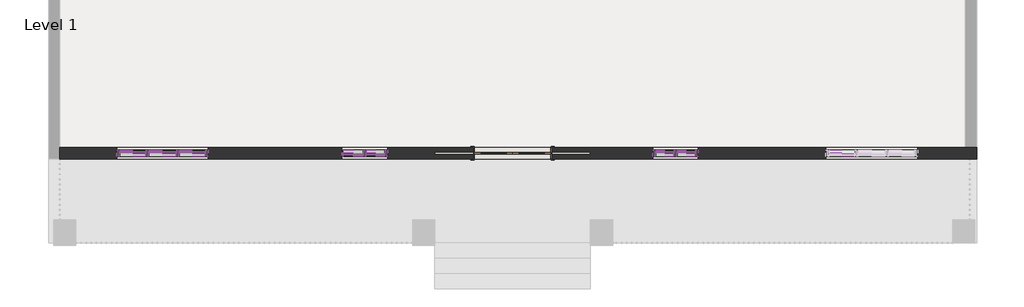
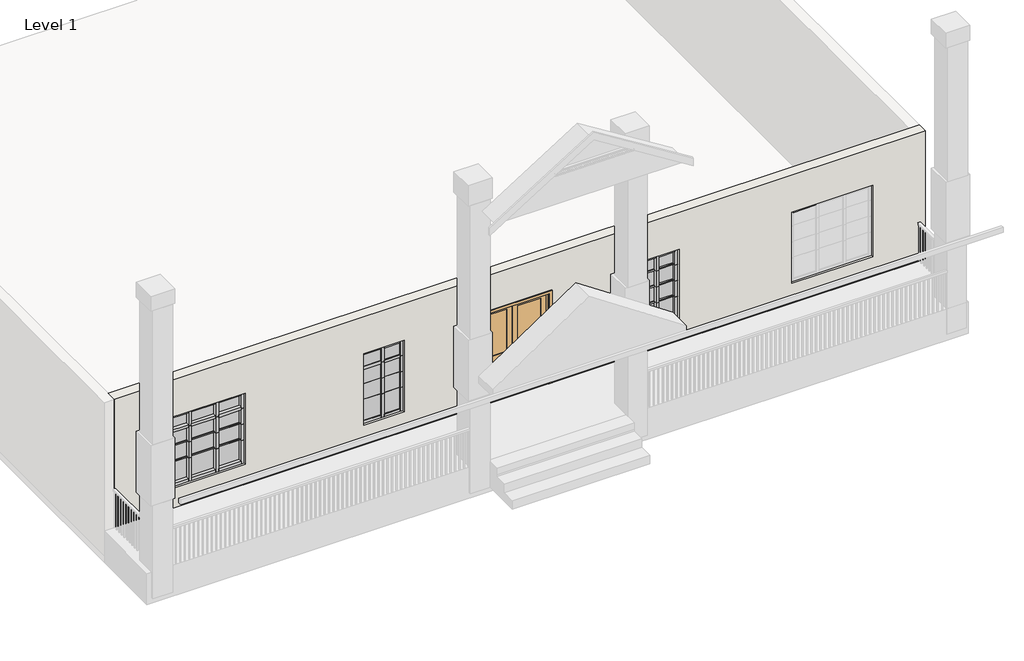
# One storey, part 1 of 3: 79 members, 28 plates, 1 door, 1 wall.
"""IFC4 building model written with IfcOpenShell, lengths in millimetres."""

from ifc_helpers import new_model, si_unit, origin, place, context, project, spatial, faceted_brep, transform, mapped, element, save
from components import door_7a66d0d1, member_34aa1075, member_9625144b, member_80fbcd94, member_5d13e7fd, member_2344d604, member_b1407fb7, member_31f2b2ad, member_0b7646a3, member_bc554fa6, member_aaa03826, member_0a1a1ade, member_a980948f, member_03a502dc, member_dfe75557, member_50cacee6, member_1ad5418d, member_843225dc, member_6103f85b, member_af2f84b9, member_d2340509, member_8fd572c7, member_8d9b4452, member_6f432376, system_panel_glazed_6026b5c4, system_panel_glazed_0f474f61, system_panel_glazed_5422c98d, system_panel_glazed_c61bacb6, system_panel_glazed_055f9577, system_panel_glazed_5ecf2d74, system_panel_glazed_969e6b50, system_panel_glazed_86de8a05, system_panel_glazed_a58f4d23, system_panel_glazed_6b1abce8, system_panel_glazed_499f07c7, system_panel_glazed_73771f90, system_panel_glazed_6a2c27ee, system_panel_glazed_d5759347, system_panel_glazed_b1e52c84, system_panel_glazed_6ee44b12, system_panel_glazed_6c61ac18, system_panel_glazed_c76c6b52, system_panel_glazed_5d34ab6a

model = new_model("IFC4")

# Units and contexts
model_context = context("Model", 3, world=origin())
ifc_project = project(units=[si_unit("LENGTHUNIT", "METRE", prefix="MILLI")], contexts=[model_context])

# Site, building, storey
site = spatial("IfcSite", under=ifc_project)
building = spatial("IfcBuilding", under=site)
storey = spatial("IfcBuildingStorey", under=building, Name="Level 1", Elevation=0.0)

# Door
placement = place(None, origin())
door_shape = door_7a66d0d1(model_context)
element("IfcDoor", 1, ObjectType="Door-Interior-Double-Pocket-2_Panel-Wood : 60\" x 84\"", at=placement, inside=storey, context=model_context, shape_type="MappedRepresentation", body=[
    mapped(door_shape, transform((-512.1420659, -6986.1878342, 609.6), x_axis=(1.0, 0.0, 0.0), y_axis=(0.0, 1.0, 0.0), z_axis=(0.0, 0.0, 1.0))),
])

# Members
member_shape = member_34aa1075(model_context)
element("IfcMember", 2, ObjectType="Rectangular Mullion : 1\" Square", at=placement, inside=storey, context=model_context, shape_type="MappedRepresentation", body=[
    mapped(member_shape, transform((-3917.6050805, -6986.1878342, 1631.95), x_axis=(-1.0, 0.0, 0.0), y_axis=(0.0, 1.0, 0.0), z_axis=(0.0, 0.0, -1.0))),
])
member_2_shape = member_9625144b(model_context)
element("IfcMember", 3, ObjectType="Rectangular Mullion : 1\" Square", at=placement, inside=storey, context=model_context, shape_type="MappedRepresentation", body=[
    mapped(member_2_shape, transform((-6646.2420659, -6986.1878342, 2006.6), x_axis=(0.0, 0.0, 1.0), y_axis=(0.0, -1.0, 0.0), z_axis=(1.0, 0.0, 0.0))),
])
element("IfcMember", 4, ObjectType="Rectangular Mullion : 1\" Square", at=placement, inside=storey, context=model_context, shape_type="MappedRepresentation", body=[
    mapped(member_2_shape, transform((-7833.6920659, -6986.1878342, 2006.6), x_axis=(0.0, 0.0, 1.0), y_axis=(0.0, -1.0, 0.0), z_axis=(1.0, 0.0, 0.0))),
])
element("IfcMember", 5, ObjectType="Rectangular Mullion : 1\" Square", at=placement, inside=storey, context=model_context, shape_type="MappedRepresentation", body=[
    mapped(member_2_shape, transform((-6646.2420659, -6986.1878342, 1625.6), x_axis=(0.0, 0.0, 1.0), y_axis=(0.0, -1.0, 0.0), z_axis=(1.0, 0.0, 0.0))),
])
element("IfcMember", 6, ObjectType="Rectangular Mullion : 1\" Square", at=placement, inside=storey, context=model_context, shape_type="MappedRepresentation", body=[
    mapped(member_2_shape, transform((-7833.6920659, -6986.1878342, 1625.6), x_axis=(0.0, 0.0, 1.0), y_axis=(0.0, -1.0, 0.0), z_axis=(1.0, 0.0, 0.0))),
])
element("IfcMember", 7, ObjectType="Rectangular Mullion : 1\" Square", at=placement, inside=storey, context=model_context, shape_type="MappedRepresentation", body=[
    mapped(member_2_shape, transform((5799.7579341, -6986.1878342, 2006.6), x_axis=(0.0, 0.0, 1.0), y_axis=(0.0, 1.0, 0.0), z_axis=(-1.0, 0.0, 0.0))),
])
element("IfcMember", 8, ObjectType="Rectangular Mullion : 1\" Square", at=placement, inside=storey, context=model_context, shape_type="MappedRepresentation", body=[
    mapped(member_2_shape, transform((5799.7579341, -6986.1878342, 1625.6), x_axis=(0.0, 0.0, 1.0), y_axis=(0.0, 1.0, 0.0), z_axis=(-1.0, 0.0, 0.0))),
])
element("IfcMember", 9, ObjectType="Rectangular Mullion : 1\" Square", at=placement, inside=storey, context=model_context, shape_type="MappedRepresentation", body=[
    mapped(member_2_shape, transform((5799.7579341, -6986.1878342, 2387.6), x_axis=(0.0, 0.0, 1.0), y_axis=(0.0, 1.0, 0.0), z_axis=(-1.0, 0.0, 0.0))),
])
member_3_shape = member_80fbcd94(model_context)
element("IfcMember", 10, ObjectType="Rectangular Mullion : 1\" Square", at=placement, inside=storey, context=model_context, shape_type="MappedRepresentation", body=[
    mapped(member_3_shape, transform((-7224.0920659, -6986.1878342, 2006.6), x_axis=(0.0, 0.0, 1.0), y_axis=(0.0, -1.0, 0.0), z_axis=(1.0, 0.0, 0.0))),
])
element("IfcMember", 11, ObjectType="Rectangular Mullion : 1\" Square", at=placement, inside=storey, context=model_context, shape_type="MappedRepresentation", body=[
    mapped(member_3_shape, transform((-7224.0920659, -6986.1878342, 1625.6), x_axis=(0.0, 0.0, 1.0), y_axis=(0.0, -1.0, 0.0), z_axis=(1.0, 0.0, 0.0))),
])
member_4_shape = member_5d13e7fd(model_context)
element("IfcMember", 12, ObjectType="Rectangular Mullion : 1\" Square", at=placement, inside=storey, context=model_context, shape_type="MappedRepresentation", body=[
    mapped(member_4_shape, transform((-3892.2050805, -6986.1878342, 2006.6), x_axis=(0.0, 0.0, 1.0), y_axis=(0.0, 1.0, 0.0), z_axis=(-1.0, 0.0, 0.0))),
])
element("IfcMember", 13, ObjectType="Rectangular Mullion : 1\" Square", at=placement, inside=storey, context=model_context, shape_type="MappedRepresentation", body=[
    mapped(member_4_shape, transform((-3892.2050805, -6986.1878342, 1631.95), x_axis=(0.0, 0.0, 1.0), y_axis=(0.0, 1.0, 0.0), z_axis=(-1.0, 0.0, 0.0))),
])
member_5_shape = member_2344d604(model_context)
element("IfcMember", 14, ObjectType="Rectangular Mullion : 1\" Square", at=placement, inside=storey, context=model_context, shape_type="MappedRepresentation", body=[
    mapped(member_5_shape, transform((-3428.6550805, -6986.1878342, 2006.6), x_axis=(0.0, 0.0, 1.0), y_axis=(0.0, 1.0, 0.0), z_axis=(-1.0, 0.0, 0.0))),
])
element("IfcMember", 15, ObjectType="Rectangular Mullion : 1\" Square", at=placement, inside=storey, context=model_context, shape_type="MappedRepresentation", body=[
    mapped(member_5_shape, transform((-3428.6550805, -6986.1878342, 1631.95), x_axis=(0.0, 0.0, 1.0), y_axis=(0.0, 1.0, 0.0), z_axis=(-1.0, 0.0, 0.0))),
])
element("IfcMember", 16, ObjectType="Rectangular Mullion : 1\" Square", at=placement, inside=storey, context=model_context, shape_type="MappedRepresentation", body=[
    mapped(member_5_shape, transform((3130.8949195, -6986.1878342, 2387.6), x_axis=(0.0, 0.0, 1.0), y_axis=(0.0, -1.0, 0.0), z_axis=(1.0, 0.0, 0.0))),
])
element("IfcMember", 17, ObjectType="Rectangular Mullion : 1\" Square", at=placement, inside=storey, context=model_context, shape_type="MappedRepresentation", body=[
    mapped(member_5_shape, transform((2705.4449195, -6986.1878342, 2387.6), x_axis=(0.0, 0.0, 1.0), y_axis=(0.0, -1.0, 0.0), z_axis=(1.0, 0.0, 0.0))),
])
element("IfcMember", 18, ObjectType="Rectangular Mullion : 1\" Square", at=placement, inside=storey, context=model_context, shape_type="MappedRepresentation", body=[
    mapped(member_5_shape, transform((3130.8949195, -6986.1878342, 2006.6), x_axis=(0.0, 0.0, 1.0), y_axis=(0.0, -1.0, 0.0), z_axis=(1.0, 0.0, 0.0))),
])
element("IfcMember", 19, ObjectType="Rectangular Mullion : 1\" Square", at=placement, inside=storey, context=model_context, shape_type="MappedRepresentation", body=[
    mapped(member_5_shape, transform((2705.4449195, -6986.1878342, 2006.6), x_axis=(0.0, 0.0, 1.0), y_axis=(0.0, -1.0, 0.0), z_axis=(1.0, 0.0, 0.0))),
])
element("IfcMember", 20, ObjectType="Rectangular Mullion : 1\" Square", at=placement, inside=storey, context=model_context, shape_type="MappedRepresentation", body=[
    mapped(member_5_shape, transform((3130.8949195, -6986.1878342, 1625.6), x_axis=(0.0, 0.0, 1.0), y_axis=(0.0, -1.0, 0.0), z_axis=(1.0, 0.0, 0.0))),
])
element("IfcMember", 21, ObjectType="Rectangular Mullion : 1\" Square", at=placement, inside=storey, context=model_context, shape_type="MappedRepresentation", body=[
    mapped(member_5_shape, transform((2705.4449195, -6986.1878342, 1625.6), x_axis=(0.0, 0.0, 1.0), y_axis=(0.0, -1.0, 0.0), z_axis=(1.0, 0.0, 0.0))),
])
member_6_shape = member_b1407fb7(model_context)
element("IfcMember", 22, ObjectType="Rectangular Mullion : 1\" Square", at=placement, inside=storey, context=model_context, shape_type="MappedRepresentation", body=[
    mapped(member_6_shape, transform((-3917.6050805, -6986.1878342, 2006.6), x_axis=(-1.0, 0.0, 0.0), y_axis=(0.0, 1.0, 0.0), z_axis=(0.0, 0.0, -1.0))),
])
element("IfcMember", 23, ObjectType="Rectangular Mullion : 1\" Square", at=placement, inside=storey, context=model_context, shape_type="MappedRepresentation", body=[
    mapped(member_6_shape, transform((-3917.6050805, -6986.1878342, 2387.6), x_axis=(-1.0, 0.0, 0.0), y_axis=(0.0, 1.0, 0.0), z_axis=(0.0, 0.0, -1.0))),
])
member_7_shape = member_31f2b2ad(model_context)
element("IfcMember", 24, ObjectType="Rectangular Mullion : 1\" Square", at=placement, inside=storey, context=model_context, shape_type="MappedRepresentation", body=[
    mapped(member_7_shape, transform((-3917.6050805, -6986.1878342, 1066.8), x_axis=(-1.0, 0.0, 0.0), y_axis=(0.0, 1.0, 0.0), z_axis=(0.0, 0.0, -1.0))),
])
member_8_shape = member_0b7646a3(model_context)
element("IfcMember", 25, ObjectType="Rectangular Mullion : 2.5\" x 5\" rectangular", at=placement, inside=storey, context=model_context, shape_type="MappedRepresentation", body=[
    mapped(member_8_shape, transform((-6646.2420659, -6986.1878342, 2768.6), x_axis=(0.0, 0.0, 1.0), y_axis=(0.0, -1.0, 0.0), z_axis=(1.0, 0.0, 0.0))),
])
element("IfcMember", 26, ObjectType="Rectangular Mullion : 2.5\" x 5\" rectangular", at=placement, inside=storey, context=model_context, shape_type="MappedRepresentation", body=[
    mapped(member_8_shape, transform((-7833.6920659, -6986.1878342, 2768.6), x_axis=(0.0, 0.0, 1.0), y_axis=(0.0, -1.0, 0.0), z_axis=(1.0, 0.0, 0.0))),
])
element("IfcMember", 27, ObjectType="Rectangular Mullion : 2.5\" x 5\" rectangular", at=placement, inside=storey, context=model_context, shape_type="MappedRepresentation", body=[
    mapped(member_8_shape, transform((5799.7579341, -6986.1878342, 2768.6), x_axis=(0.0, 0.0, 1.0), y_axis=(0.0, 1.0, 0.0), z_axis=(-1.0, 0.0, 0.0))),
])
element("IfcMember", 28, ObjectType="Rectangular Mullion : 2.5\" x 5\" rectangular", at=placement, inside=storey, context=model_context, shape_type="MappedRepresentation", body=[
    mapped(member_8_shape, transform((-8348.0420659, -6986.1878342, 1066.8), x_axis=(0.0, 0.0, -1.0), y_axis=(0.0, -1.0, 0.0), z_axis=(-1.0, 0.0, 0.0))),
])
element("IfcMember", 29, ObjectType="Rectangular Mullion : 2.5\" x 5\" rectangular", at=placement, inside=storey, context=model_context, shape_type="MappedRepresentation", body=[
    mapped(member_8_shape, transform((-7160.5920659, -6986.1878342, 1066.8), x_axis=(0.0, 0.0, -1.0), y_axis=(0.0, -1.0, 0.0), z_axis=(-1.0, 0.0, 0.0))),
])
member_9_shape = member_bc554fa6(model_context)
element("IfcMember", 30, ObjectType="Rectangular Mullion : 2.5\" x 5\" rectangular", at=placement, inside=storey, context=model_context, shape_type="MappedRepresentation", body=[
    mapped(member_9_shape, transform((-7801.9420659, -6986.1878342, 1066.8), x_axis=(1.0, 0.0, 0.0), y_axis=(0.0, -1.0, 0.0), z_axis=(0.0, 0.0, -1.0))),
])
element("IfcMember", 31, ObjectType="Rectangular Mullion : 2.5\" x 5\" rectangular", at=placement, inside=storey, context=model_context, shape_type="MappedRepresentation", body=[
    mapped(member_9_shape, transform((-7192.3420659, -6986.1878342, 1066.8), x_axis=(1.0, 0.0, 0.0), y_axis=(0.0, -1.0, 0.0), z_axis=(0.0, 0.0, -1.0))),
])
element("IfcMember", 32, ObjectType="Rectangular Mullion : 2.5\" x 5\" rectangular", at=placement, inside=storey, context=model_context, shape_type="MappedRepresentation", body=[
    mapped(member_9_shape, transform((2737.1949195, -6986.1878342, 1066.8), x_axis=(1.0, 0.0, 0.0), y_axis=(0.0, -1.0, 0.0), z_axis=(0.0, 0.0, -1.0))),
])
member_10_shape = member_aaa03826(model_context)
element("IfcMember", 33, ObjectType="Rectangular Mullion : 2.5\" x 5\" rectangular", at=placement, inside=storey, context=model_context, shape_type="MappedRepresentation", body=[
    mapped(member_10_shape, transform((-7833.6920659, -6986.1878342, 2387.6), x_axis=(0.0, 0.0, 1.0), y_axis=(0.0, -1.0, 0.0), z_axis=(1.0, 0.0, 0.0))),
])
element("IfcMember", 34, ObjectType="Rectangular Mullion : 2.5\" x 5\" rectangular", at=placement, inside=storey, context=model_context, shape_type="MappedRepresentation", body=[
    mapped(member_10_shape, transform((-6646.2420659, -6986.1878342, 2387.6), x_axis=(0.0, 0.0, 1.0), y_axis=(0.0, -1.0, 0.0), z_axis=(1.0, 0.0, 0.0))),
])
member_11_shape = member_0a1a1ade(model_context)
element("IfcMember", 35, ObjectType="Rectangular Mullion : 2.5\" x 5\" rectangular", at=placement, inside=storey, context=model_context, shape_type="MappedRepresentation", body=[
    mapped(member_11_shape, transform((-7224.0920659, -6986.1878342, 2387.6), x_axis=(0.0, 0.0, 1.0), y_axis=(0.0, -1.0, 0.0), z_axis=(1.0, 0.0, 0.0))),
])
member_12_shape = member_a980948f(model_context)
element("IfcMember", 36, ObjectType="Rectangular Mullion : 2.5\" x 5\" rectangular", at=placement, inside=storey, context=model_context, shape_type="MappedRepresentation", body=[
    mapped(member_12_shape, transform((-7770.1920659, -6986.1878342, 1066.8), x_axis=(0.0, 0.0, -1.0), y_axis=(0.0, -1.0, 0.0), z_axis=(-1.0, 0.0, 0.0))),
])
element("IfcMember", 37, ObjectType="Rectangular Mullion : 2.5\" x 5\" rectangular", at=placement, inside=storey, context=model_context, shape_type="MappedRepresentation", body=[
    mapped(member_12_shape, transform((-7224.0920659, -6986.1878342, 2768.6), x_axis=(0.0, 0.0, 1.0), y_axis=(0.0, -1.0, 0.0), z_axis=(1.0, 0.0, 0.0))),
])
member_13_shape = member_03a502dc(model_context)
element("IfcMember", 38, ObjectType="Rectangular Mullion : 2.5\" x 5\" rectangular", at=placement, inside=storey, context=model_context, shape_type="MappedRepresentation", body=[
    mapped(member_13_shape, transform((-7801.9420659, -6986.1878342, 2387.6), x_axis=(1.0, 0.0, 0.0), y_axis=(0.0, -1.0, 0.0), z_axis=(0.0, 0.0, -1.0))),
])
element("IfcMember", 39, ObjectType="Rectangular Mullion : 2.5\" x 5\" rectangular", at=placement, inside=storey, context=model_context, shape_type="MappedRepresentation", body=[
    mapped(member_13_shape, transform((-7192.3420659, -6986.1878342, 2387.6), x_axis=(1.0, 0.0, 0.0), y_axis=(0.0, -1.0, 0.0), z_axis=(0.0, 0.0, -1.0))),
])
element("IfcMember", 40, ObjectType="Rectangular Mullion : 2.5\" x 5\" rectangular", at=placement, inside=storey, context=model_context, shape_type="MappedRepresentation", body=[
    mapped(member_13_shape, transform((-3460.4050805, -6986.1878342, 2387.6), x_axis=(-1.0, 0.0, 0.0), y_axis=(0.0, 1.0, 0.0), z_axis=(0.0, 0.0, -1.0))),
])
element("IfcMember", 41, ObjectType="Rectangular Mullion : 2.5\" x 5\" rectangular", at=placement, inside=storey, context=model_context, shape_type="MappedRepresentation", body=[
    mapped(member_13_shape, transform((2737.1949195, -6986.1878342, 2387.6), x_axis=(1.0, 0.0, 0.0), y_axis=(0.0, -1.0, 0.0), z_axis=(0.0, 0.0, -1.0))),
])
element("IfcMember", 42, ObjectType="Rectangular Mullion : 2.5\" x 5\" rectangular", at=placement, inside=storey, context=model_context, shape_type="MappedRepresentation", body=[
    mapped(member_13_shape, transform((-7801.9420659, -6986.1878342, 2006.6), x_axis=(1.0, 0.0, 0.0), y_axis=(0.0, -1.0, 0.0), z_axis=(0.0, 0.0, -1.0))),
])
element("IfcMember", 43, ObjectType="Rectangular Mullion : 2.5\" x 5\" rectangular", at=placement, inside=storey, context=model_context, shape_type="MappedRepresentation", body=[
    mapped(member_13_shape, transform((-7801.9420659, -6986.1878342, 1625.6), x_axis=(1.0, 0.0, 0.0), y_axis=(0.0, -1.0, 0.0), z_axis=(0.0, 0.0, -1.0))),
])
element("IfcMember", 44, ObjectType="Rectangular Mullion : 2.5\" x 5\" rectangular", at=placement, inside=storey, context=model_context, shape_type="MappedRepresentation", body=[
    mapped(member_13_shape, transform((-7192.3420659, -6986.1878342, 2006.6), x_axis=(1.0, 0.0, 0.0), y_axis=(0.0, -1.0, 0.0), z_axis=(0.0, 0.0, -1.0))),
])
element("IfcMember", 45, ObjectType="Rectangular Mullion : 2.5\" x 5\" rectangular", at=placement, inside=storey, context=model_context, shape_type="MappedRepresentation", body=[
    mapped(member_13_shape, transform((-7192.3420659, -6986.1878342, 1625.6), x_axis=(1.0, 0.0, 0.0), y_axis=(0.0, -1.0, 0.0), z_axis=(0.0, 0.0, -1.0))),
])
element("IfcMember", 46, ObjectType="Rectangular Mullion : 2.5\" x 5\" rectangular", at=placement, inside=storey, context=model_context, shape_type="MappedRepresentation", body=[
    mapped(member_13_shape, transform((-3460.4050805, -6986.1878342, 2006.6), x_axis=(-1.0, 0.0, 0.0), y_axis=(0.0, 1.0, 0.0), z_axis=(0.0, 0.0, -1.0))),
])
element("IfcMember", 47, ObjectType="Rectangular Mullion : 2.5\" x 5\" rectangular", at=placement, inside=storey, context=model_context, shape_type="MappedRepresentation", body=[
    mapped(member_13_shape, transform((2737.1949195, -6986.1878342, 2006.6), x_axis=(1.0, 0.0, 0.0), y_axis=(0.0, -1.0, 0.0), z_axis=(0.0, 0.0, -1.0))),
])
element("IfcMember", 48, ObjectType="Rectangular Mullion : 2.5\" x 5\" rectangular", at=placement, inside=storey, context=model_context, shape_type="MappedRepresentation", body=[
    mapped(member_13_shape, transform((2737.1949195, -6986.1878342, 1625.6), x_axis=(1.0, 0.0, 0.0), y_axis=(0.0, -1.0, 0.0), z_axis=(0.0, 0.0, -1.0))),
])
member_14_shape = member_dfe75557(model_context)
element("IfcMember", 49, ObjectType="Rectangular Mullion : 2.5\" x 5\" rectangular", at=placement, inside=storey, context=model_context, shape_type="MappedRepresentation", body=[
    mapped(member_14_shape, transform((-8411.5420659, -6986.1878342, 2768.6), x_axis=(-1.0, 0.0, 0.0), y_axis=(0.0, -1.0, 0.0), z_axis=(0.0, 0.0, 1.0))),
])
element("IfcMember", 50, ObjectType="Rectangular Mullion : 2.5\" x 5\" rectangular", at=placement, inside=storey, context=model_context, shape_type="MappedRepresentation", body=[
    mapped(member_14_shape, transform((-3003.2050805, -6986.1878342, 2768.6), x_axis=(1.0, 0.0, 0.0), y_axis=(0.0, 1.0, 0.0), z_axis=(0.0, 0.0, 1.0))),
])
element("IfcMember", 51, ObjectType="Rectangular Mullion : 2.5\" x 5\" rectangular", at=placement, inside=storey, context=model_context, shape_type="MappedRepresentation", body=[
    mapped(member_14_shape, transform((2279.9949195, -6986.1878342, 2768.6), x_axis=(-1.0, 0.0, 0.0), y_axis=(0.0, -1.0, 0.0), z_axis=(0.0, 0.0, 1.0))),
])
member_15_shape = member_50cacee6(model_context)
element("IfcMember", 52, ObjectType="Rectangular Mullion : 2.5\" x 5\" rectangular", at=placement, inside=storey, context=model_context, shape_type="MappedRepresentation", body=[
    mapped(member_15_shape, transform((-6582.7420659, -6986.1878342, 1066.8), x_axis=(1.0, 0.0, 0.0), y_axis=(0.0, -1.0, 0.0), z_axis=(0.0, 0.0, -1.0))),
])
element("IfcMember", 53, ObjectType="Rectangular Mullion : 2.5\" x 5\" rectangular", at=placement, inside=storey, context=model_context, shape_type="MappedRepresentation", body=[
    mapped(member_15_shape, transform((3194.3949195, -6986.1878342, 1066.8), x_axis=(1.0, 0.0, 0.0), y_axis=(0.0, -1.0, 0.0), z_axis=(0.0, 0.0, -1.0))),
])
element("IfcMember", 54, ObjectType="Rectangular Mullion : 2.5\" x 5\" rectangular", at=placement, inside=storey, context=model_context, shape_type="MappedRepresentation", body=[
    mapped(member_14_shape, transform((-6582.7420659, -6986.1878342, 2387.6), x_axis=(1.0, 0.0, 0.0), y_axis=(0.0, -1.0, 0.0), z_axis=(0.0, 0.0, -1.0))),
])
element("IfcMember", 55, ObjectType="Rectangular Mullion : 2.5\" x 5\" rectangular", at=placement, inside=storey, context=model_context, shape_type="MappedRepresentation", body=[
    mapped(member_14_shape, transform((3194.3949195, -6986.1878342, 2387.6), x_axis=(1.0, 0.0, 0.0), y_axis=(0.0, -1.0, 0.0), z_axis=(0.0, 0.0, -1.0))),
])
element("IfcMember", 56, ObjectType="Rectangular Mullion : 2.5\" x 5\" rectangular", at=placement, inside=storey, context=model_context, shape_type="MappedRepresentation", body=[
    mapped(member_14_shape, transform((-6582.7420659, -6986.1878342, 2006.6), x_axis=(1.0, 0.0, 0.0), y_axis=(0.0, -1.0, 0.0), z_axis=(0.0, 0.0, -1.0))),
])
element("IfcMember", 57, ObjectType="Rectangular Mullion : 2.5\" x 5\" rectangular", at=placement, inside=storey, context=model_context, shape_type="MappedRepresentation", body=[
    mapped(member_14_shape, transform((-6582.7420659, -6986.1878342, 1625.6), x_axis=(1.0, 0.0, 0.0), y_axis=(0.0, -1.0, 0.0), z_axis=(0.0, 0.0, -1.0))),
])
element("IfcMember", 58, ObjectType="Rectangular Mullion : 2.5\" x 5\" rectangular", at=placement, inside=storey, context=model_context, shape_type="MappedRepresentation", body=[
    mapped(member_14_shape, transform((3194.3949195, -6986.1878342, 2006.6), x_axis=(1.0, 0.0, 0.0), y_axis=(0.0, -1.0, 0.0), z_axis=(0.0, 0.0, -1.0))),
])
element("IfcMember", 59, ObjectType="Rectangular Mullion : 2.5\" x 5\" rectangular", at=placement, inside=storey, context=model_context, shape_type="MappedRepresentation", body=[
    mapped(member_14_shape, transform((3194.3949195, -6986.1878342, 1625.6), x_axis=(1.0, 0.0, 0.0), y_axis=(0.0, -1.0, 0.0), z_axis=(0.0, 0.0, -1.0))),
])
element("IfcMember", 60, ObjectType="Rectangular Mullion : 2.5\" x 5\" rectangular", at=placement, inside=storey, context=model_context, shape_type="MappedRepresentation", body=[
    mapped(member_14_shape, transform((-8411.5420659, -6986.1878342, 2387.6), x_axis=(-1.0, 0.0, 0.0), y_axis=(0.0, -1.0, 0.0), z_axis=(0.0, 0.0, 1.0))),
])
element("IfcMember", 61, ObjectType="Rectangular Mullion : 2.5\" x 5\" rectangular", at=placement, inside=storey, context=model_context, shape_type="MappedRepresentation", body=[
    mapped(member_14_shape, transform((-8411.5420659, -6986.1878342, 2006.6), x_axis=(-1.0, 0.0, 0.0), y_axis=(0.0, -1.0, 0.0), z_axis=(0.0, 0.0, 1.0))),
])
element("IfcMember", 62, ObjectType="Rectangular Mullion : 2.5\" x 5\" rectangular", at=placement, inside=storey, context=model_context, shape_type="MappedRepresentation", body=[
    mapped(member_14_shape, transform((-3003.2050805, -6986.1878342, 2387.6), x_axis=(1.0, 0.0, 0.0), y_axis=(0.0, 1.0, 0.0), z_axis=(0.0, 0.0, 1.0))),
])
element("IfcMember", 63, ObjectType="Rectangular Mullion : 2.5\" x 5\" rectangular", at=placement, inside=storey, context=model_context, shape_type="MappedRepresentation", body=[
    mapped(member_14_shape, transform((2279.9949195, -6986.1878342, 2387.6), x_axis=(-1.0, 0.0, 0.0), y_axis=(0.0, -1.0, 0.0), z_axis=(0.0, 0.0, 1.0))),
])
element("IfcMember", 64, ObjectType="Rectangular Mullion : 2.5\" x 5\" rectangular", at=placement, inside=storey, context=model_context, shape_type="MappedRepresentation", body=[
    mapped(member_14_shape, transform((2279.9949195, -6986.1878342, 2006.6), x_axis=(-1.0, 0.0, 0.0), y_axis=(0.0, -1.0, 0.0), z_axis=(0.0, 0.0, 1.0))),
])
element("IfcMember", 65, ObjectType="Rectangular Mullion : 2.5\" x 5\" rectangular", at=placement, inside=storey, context=model_context, shape_type="MappedRepresentation", body=[
    mapped(member_15_shape, transform((-8411.5420659, -6986.1878342, 1625.6), x_axis=(-1.0, 0.0, 0.0), y_axis=(0.0, -1.0, 0.0), z_axis=(0.0, 0.0, 1.0))),
])
element("IfcMember", 66, ObjectType="Rectangular Mullion : 2.5\" x 5\" rectangular", at=placement, inside=storey, context=model_context, shape_type="MappedRepresentation", body=[
    mapped(member_15_shape, transform((2279.9949195, -6986.1878342, 1625.6), x_axis=(-1.0, 0.0, 0.0), y_axis=(0.0, -1.0, 0.0), z_axis=(0.0, 0.0, 1.0))),
])
member_16_shape = member_1ad5418d(model_context)
element("IfcMember", 67, ObjectType="Rectangular Mullion : 2.5\" x 5\" rectangular", at=placement, inside=storey, context=model_context, shape_type="MappedRepresentation", body=[
    mapped(member_16_shape, transform((-3892.2050805, -6986.1878342, 2768.6), x_axis=(0.0, 0.0, 1.0), y_axis=(0.0, 1.0, 0.0), z_axis=(-1.0, 0.0, 0.0))),
])
member_17_shape = member_843225dc(model_context)
element("IfcMember", 68, ObjectType="Rectangular Mullion : 2.5\" x 5\" rectangular", at=placement, inside=storey, context=model_context, shape_type="MappedRepresentation", body=[
    mapped(member_17_shape, transform((-3066.7050805, -6986.1878342, 1066.8), x_axis=(0.0, 0.0, -1.0), y_axis=(0.0, 1.0, 0.0), z_axis=(1.0, 0.0, 0.0))),
])
element("IfcMember", 69, ObjectType="Rectangular Mullion : 2.5\" x 5\" rectangular", at=placement, inside=storey, context=model_context, shape_type="MappedRepresentation", body=[
    mapped(member_17_shape, transform((2343.4949195, -6986.1878342, 1066.8), x_axis=(0.0, 0.0, -1.0), y_axis=(0.0, -1.0, 0.0), z_axis=(-1.0, 0.0, 0.0))),
])
element("IfcMember", 70, ObjectType="Rectangular Mullion : 2.5\" x 5\" rectangular", at=placement, inside=storey, context=model_context, shape_type="MappedRepresentation", body=[
    mapped(member_17_shape, transform((2768.9449195, -6986.1878342, 1066.8), x_axis=(0.0, 0.0, -1.0), y_axis=(0.0, -1.0, 0.0), z_axis=(-1.0, 0.0, 0.0))),
])
member_18_shape = member_6103f85b(model_context)
element("IfcMember", 71, ObjectType="Rectangular Mullion : 2.5\" x 5\" rectangular", at=placement, inside=storey, context=model_context, shape_type="MappedRepresentation", body=[
    mapped(member_18_shape, transform((-3460.4050805, -6986.1878342, 1066.8), x_axis=(-1.0, 0.0, 0.0), y_axis=(0.0, 1.0, 0.0), z_axis=(0.0, 0.0, -1.0))),
])
member_19_shape = member_af2f84b9(model_context)
element("IfcMember", 72, ObjectType="Rectangular Mullion : 2.5\" x 5\" rectangular", at=placement, inside=storey, context=model_context, shape_type="MappedRepresentation", body=[
    mapped(member_19_shape, transform((-3428.6550805, -6986.1878342, 2387.6), x_axis=(0.0, 0.0, 1.0), y_axis=(0.0, 1.0, 0.0), z_axis=(-1.0, 0.0, 0.0))),
])
member_20_shape = member_d2340509(model_context)
element("IfcMember", 73, ObjectType="Rectangular Mullion : 2.5\" x 5\" rectangular", at=placement, inside=storey, context=model_context, shape_type="MappedRepresentation", body=[
    mapped(member_20_shape, transform((-3892.2050805, -6986.1878342, 2387.6), x_axis=(0.0, 0.0, 1.0), y_axis=(0.0, 1.0, 0.0), z_axis=(-1.0, 0.0, 0.0))),
])
element("IfcMember", 74, ObjectType="Rectangular Mullion : 2.5\" x 5\" rectangular", at=placement, inside=storey, context=model_context, shape_type="MappedRepresentation", body=[
    mapped(member_16_shape, transform((-3492.1550805, -6986.1878342, 1066.8), x_axis=(0.0, 0.0, -1.0), y_axis=(0.0, 1.0, 0.0), z_axis=(1.0, 0.0, 0.0))),
])
element("IfcMember", 75, ObjectType="Rectangular Mullion : 2.5\" x 5\" rectangular", at=placement, inside=storey, context=model_context, shape_type="MappedRepresentation", body=[
    mapped(member_17_shape, transform((-3428.6550805, -6986.1878342, 2768.6), x_axis=(0.0, 0.0, 1.0), y_axis=(0.0, 1.0, 0.0), z_axis=(-1.0, 0.0, 0.0))),
])
element("IfcMember", 76, ObjectType="Rectangular Mullion : 2.5\" x 5\" rectangular", at=placement, inside=storey, context=model_context, shape_type="MappedRepresentation", body=[
    mapped(member_17_shape, transform((3130.8949195, -6986.1878342, 2768.6), x_axis=(0.0, 0.0, 1.0), y_axis=(0.0, -1.0, 0.0), z_axis=(1.0, 0.0, 0.0))),
])
element("IfcMember", 77, ObjectType="Rectangular Mullion : 2.5\" x 5\" rectangular", at=placement, inside=storey, context=model_context, shape_type="MappedRepresentation", body=[
    mapped(member_17_shape, transform((2705.4449195, -6986.1878342, 2768.6), x_axis=(0.0, 0.0, 1.0), y_axis=(0.0, -1.0, 0.0), z_axis=(1.0, 0.0, 0.0))),
])
member_21_shape = member_8fd572c7(model_context)
element("IfcMember", 78, ObjectType="Rectangular Mullion : 2.5\" x 5\" rectangular", at=placement, inside=storey, context=model_context, shape_type="MappedRepresentation", body=[
    mapped(member_21_shape, transform((-3460.4050805, -6986.1878342, 1631.95), x_axis=(-1.0, 0.0, 0.0), y_axis=(0.0, 1.0, 0.0), z_axis=(0.0, 0.0, -1.0))),
])
member_22_shape = member_8d9b4452(model_context)
element("IfcMember", 79, ObjectType="Rectangular Mullion : 2.5\" x 5\" rectangular", at=placement, inside=storey, context=model_context, shape_type="MappedRepresentation", body=[
    mapped(member_22_shape, transform((-3003.2050805, -6986.1878342, 2006.6), x_axis=(1.0, 0.0, 0.0), y_axis=(0.0, 1.0, 0.0), z_axis=(0.0, 0.0, 1.0))),
])
member_23_shape = member_6f432376(model_context)
element("IfcMember", 80, ObjectType="Rectangular Mullion : 2.5\" x 5\" rectangular", at=placement, inside=storey, context=model_context, shape_type="MappedRepresentation", body=[
    mapped(member_23_shape, transform((-3003.2050805, -6986.1878342, 1631.95), x_axis=(1.0, 0.0, 0.0), y_axis=(0.0, 1.0, 0.0), z_axis=(0.0, 0.0, 1.0))),
])

# Plates
system_panel_glazed_shape = system_panel_glazed_6026b5c4(model_context)
element("IfcPlate", 81, ObjectType="System Panel : Glazed", at=placement, inside=storey, context=model_context, shape_type="MappedRepresentation", body=[
    mapped(system_panel_glazed_shape, transform((-8090.8670659, -6986.1878342, 1130.3), x_axis=(1.0, 0.0, 0.0), y_axis=(0.0, 1.0, 0.0), z_axis=(0.0, 0.0, 1.0))),
])
element("IfcPlate", 82, ObjectType="System Panel : Glazed", at=placement, inside=storey, context=model_context, shape_type="MappedRepresentation", body=[
    mapped(system_panel_glazed_shape, transform((-6903.4170659, -6986.1878342, 1130.3), x_axis=(1.0, 0.0, 0.0), y_axis=(0.0, 1.0, 0.0), z_axis=(0.0, 0.0, 1.0))),
])
system_panel_glazed_2_shape = system_panel_glazed_0f474f61(model_context)
element("IfcPlate", 83, ObjectType="System Panel : Glazed", at=placement, inside=storey, context=model_context, shape_type="MappedRepresentation", body=[
    mapped(system_panel_glazed_2_shape, transform((-7497.1420659, -6986.1878342, 1130.3), x_axis=(1.0, 0.0, 0.0), y_axis=(0.0, 1.0, 0.0), z_axis=(0.0, 0.0, 1.0))),
])
system_panel_glazed_3_shape = system_panel_glazed_5422c98d(model_context)
element("IfcPlate", 84, ObjectType="System Panel : Glazed", at=placement, inside=storey, context=model_context, shape_type="MappedRepresentation", body=[
    mapped(system_panel_glazed_3_shape, transform((-8090.8670659, -6986.1878342, 2419.35), x_axis=(1.0, 0.0, 0.0), y_axis=(0.0, 1.0, 0.0), z_axis=(0.0, 0.0, 1.0))),
])
element("IfcPlate", 85, ObjectType="System Panel : Glazed", at=placement, inside=storey, context=model_context, shape_type="MappedRepresentation", body=[
    mapped(system_panel_glazed_3_shape, transform((-6903.4170659, -6986.1878342, 2419.35), x_axis=(1.0, 0.0, 0.0), y_axis=(0.0, 1.0, 0.0), z_axis=(0.0, 0.0, 1.0))),
])
system_panel_glazed_4_shape = system_panel_glazed_c61bacb6(model_context)
element("IfcPlate", 86, ObjectType="System Panel : Glazed", at=placement, inside=storey, context=model_context, shape_type="MappedRepresentation", body=[
    mapped(system_panel_glazed_4_shape, transform((-7497.1420659, -6986.1878342, 2419.35), x_axis=(1.0, 0.0, 0.0), y_axis=(0.0, 1.0, 0.0), z_axis=(0.0, 0.0, 1.0))),
])
system_panel_glazed_5_shape = system_panel_glazed_055f9577(model_context)
element("IfcPlate", 87, ObjectType="System Panel : Glazed", at=placement, inside=storey, context=model_context, shape_type="MappedRepresentation", body=[
    mapped(system_panel_glazed_5_shape, transform((-8090.8670659, -6986.1878342, 2006.6), x_axis=(1.0, 0.0, 0.0), y_axis=(0.0, 1.0, 0.0), z_axis=(0.0, 0.0, 1.0))),
])
element("IfcPlate", 88, ObjectType="System Panel : Glazed", at=placement, inside=storey, context=model_context, shape_type="MappedRepresentation", body=[
    mapped(system_panel_glazed_5_shape, transform((-6903.4170659, -6986.1878342, 2006.6), x_axis=(1.0, 0.0, 0.0), y_axis=(0.0, 1.0, 0.0), z_axis=(0.0, 0.0, 1.0))),
])
system_panel_glazed_6_shape = system_panel_glazed_5ecf2d74(model_context)
element("IfcPlate", 89, ObjectType="System Panel : Glazed", at=placement, inside=storey, context=model_context, shape_type="MappedRepresentation", body=[
    mapped(system_panel_glazed_6_shape, transform((-7497.1420659, -6986.1878342, 2006.6), x_axis=(1.0, 0.0, 0.0), y_axis=(0.0, 1.0, 0.0), z_axis=(0.0, 0.0, 1.0))),
])
system_panel_glazed_7_shape = system_panel_glazed_969e6b50(model_context)
element("IfcPlate", 90, ObjectType="System Panel : Glazed", at=placement, inside=storey, context=model_context, shape_type="MappedRepresentation", body=[
    mapped(system_panel_glazed_7_shape, transform((-8090.8670659, -6986.1878342, 1625.6), x_axis=(1.0, 0.0, 0.0), y_axis=(0.0, 1.0, 0.0), z_axis=(0.0, 0.0, 1.0))),
])
element("IfcPlate", 91, ObjectType="System Panel : Glazed", at=placement, inside=storey, context=model_context, shape_type="MappedRepresentation", body=[
    mapped(system_panel_glazed_7_shape, transform((-6903.4170659, -6986.1878342, 1625.6), x_axis=(1.0, 0.0, 0.0), y_axis=(0.0, 1.0, 0.0), z_axis=(0.0, 0.0, 1.0))),
])
system_panel_glazed_8_shape = system_panel_glazed_86de8a05(model_context)
element("IfcPlate", 92, ObjectType="System Panel : Glazed", at=placement, inside=storey, context=model_context, shape_type="MappedRepresentation", body=[
    mapped(system_panel_glazed_8_shape, transform((-7497.1420659, -6986.1878342, 1625.6), x_axis=(1.0, 0.0, 0.0), y_axis=(0.0, 1.0, 0.0), z_axis=(0.0, 0.0, 1.0))),
])
system_panel_glazed_9_shape = system_panel_glazed_a58f4d23(model_context)
element("IfcPlate", 93, ObjectType="System Panel : Glazed", at=placement, inside=storey, context=model_context, shape_type="MappedRepresentation", body=[
    mapped(system_panel_glazed_9_shape, transform((-3247.6800805, -6986.1878342, 1130.3), x_axis=(-1.0, 0.0, 0.0), y_axis=(0.0, -1.0, 0.0), z_axis=(0.0, 0.0, 1.0))),
])
system_panel_glazed_10_shape = system_panel_glazed_6b1abce8(model_context)
element("IfcPlate", 94, ObjectType="System Panel : Glazed", at=placement, inside=storey, context=model_context, shape_type="MappedRepresentation", body=[
    mapped(system_panel_glazed_10_shape, transform((-3704.8800805, -6986.1878342, 1130.3), x_axis=(-1.0, 0.0, 0.0), y_axis=(0.0, -1.0, 0.0), z_axis=(0.0, 0.0, 1.0))),
])
system_panel_glazed_11_shape = system_panel_glazed_499f07c7(model_context)
element("IfcPlate", 95, ObjectType="System Panel : Glazed", at=placement, inside=storey, context=model_context, shape_type="MappedRepresentation", body=[
    mapped(system_panel_glazed_11_shape, transform((-3247.6800805, -6986.1878342, 2419.35), x_axis=(-1.0, 0.0, 0.0), y_axis=(0.0, -1.0, 0.0), z_axis=(0.0, 0.0, 1.0))),
])
system_panel_glazed_12_shape = system_panel_glazed_73771f90(model_context)
element("IfcPlate", 96, ObjectType="System Panel : Glazed", at=placement, inside=storey, context=model_context, shape_type="MappedRepresentation", body=[
    mapped(system_panel_glazed_12_shape, transform((-3704.8800805, -6986.1878342, 2419.35), x_axis=(-1.0, 0.0, 0.0), y_axis=(0.0, -1.0, 0.0), z_axis=(0.0, 0.0, 1.0))),
])
system_panel_glazed_13_shape = system_panel_glazed_6a2c27ee(model_context)
element("IfcPlate", 97, ObjectType="System Panel : Glazed", at=placement, inside=storey, context=model_context, shape_type="MappedRepresentation", body=[
    mapped(system_panel_glazed_13_shape, transform((-3247.6800805, -6986.1878342, 2006.6), x_axis=(-1.0, 0.0, 0.0), y_axis=(0.0, -1.0, 0.0), z_axis=(0.0, 0.0, 1.0))),
])
system_panel_glazed_14_shape = system_panel_glazed_d5759347(model_context)
element("IfcPlate", 98, ObjectType="System Panel : Glazed", at=placement, inside=storey, context=model_context, shape_type="MappedRepresentation", body=[
    mapped(system_panel_glazed_14_shape, transform((-3704.8800805, -6986.1878342, 2006.6), x_axis=(-1.0, 0.0, 0.0), y_axis=(0.0, -1.0, 0.0), z_axis=(0.0, 0.0, 1.0))),
])
system_panel_glazed_15_shape = system_panel_glazed_b1e52c84(model_context)
element("IfcPlate", 99, ObjectType="System Panel : Glazed", at=placement, inside=storey, context=model_context, shape_type="MappedRepresentation", body=[
    mapped(system_panel_glazed_15_shape, transform((-3247.6800805, -6986.1878342, 1631.95), x_axis=(-1.0, 0.0, 0.0), y_axis=(0.0, -1.0, 0.0), z_axis=(0.0, 0.0, 1.0))),
])
system_panel_glazed_16_shape = system_panel_glazed_6ee44b12(model_context)
element("IfcPlate", 100, ObjectType="System Panel : Glazed", at=placement, inside=storey, context=model_context, shape_type="MappedRepresentation", body=[
    mapped(system_panel_glazed_16_shape, transform((-3704.8800805, -6986.1878342, 1631.95), x_axis=(-1.0, 0.0, 0.0), y_axis=(0.0, -1.0, 0.0), z_axis=(0.0, 0.0, 1.0))),
])
system_panel_glazed_17_shape = system_panel_glazed_6c61ac18(model_context)
element("IfcPlate", 101, ObjectType="System Panel : Glazed", at=placement, inside=storey, context=model_context, shape_type="MappedRepresentation", body=[
    mapped(system_panel_glazed_17_shape, transform((2524.4699195, -6986.1878342, 1130.3), x_axis=(1.0, 0.0, 0.0), y_axis=(0.0, 1.0, 0.0), z_axis=(0.0, 0.0, 1.0))),
])
element("IfcPlate", 102, ObjectType="System Panel : Glazed", at=placement, inside=storey, context=model_context, shape_type="MappedRepresentation", body=[
    mapped(system_panel_glazed_17_shape, transform((2949.9199195, -6986.1878342, 1130.3), x_axis=(1.0, 0.0, 0.0), y_axis=(0.0, 1.0, 0.0), z_axis=(0.0, 0.0, 1.0))),
])
system_panel_glazed_18_shape = system_panel_glazed_c76c6b52(model_context)
element("IfcPlate", 103, ObjectType="System Panel : Glazed", at=placement, inside=storey, context=model_context, shape_type="MappedRepresentation", body=[
    mapped(system_panel_glazed_18_shape, transform((2524.4699195, -6986.1878342, 2387.6), x_axis=(1.0, 0.0, 0.0), y_axis=(0.0, 1.0, 0.0), z_axis=(0.0, 0.0, 1.0))),
])
element("IfcPlate", 104, ObjectType="System Panel : Glazed", at=placement, inside=storey, context=model_context, shape_type="MappedRepresentation", body=[
    mapped(system_panel_glazed_18_shape, transform((2949.9199195, -6986.1878342, 2387.6), x_axis=(1.0, 0.0, 0.0), y_axis=(0.0, 1.0, 0.0), z_axis=(0.0, 0.0, 1.0))),
])
system_panel_glazed_19_shape = system_panel_glazed_5d34ab6a(model_context)
element("IfcPlate", 105, ObjectType="System Panel : Glazed", at=placement, inside=storey, context=model_context, shape_type="MappedRepresentation", body=[
    mapped(system_panel_glazed_19_shape, transform((2524.4699195, -6986.1878342, 2006.6), x_axis=(1.0, 0.0, 0.0), y_axis=(0.0, 1.0, 0.0), z_axis=(0.0, 0.0, 1.0))),
])
element("IfcPlate", 106, ObjectType="System Panel : Glazed", at=placement, inside=storey, context=model_context, shape_type="MappedRepresentation", body=[
    mapped(system_panel_glazed_19_shape, transform((2949.9199195, -6986.1878342, 2006.6), x_axis=(1.0, 0.0, 0.0), y_axis=(0.0, 1.0, 0.0), z_axis=(0.0, 0.0, 1.0))),
])
element("IfcPlate", 107, ObjectType="System Panel : Glazed", at=placement, inside=storey, context=model_context, shape_type="MappedRepresentation", body=[
    mapped(system_panel_glazed_19_shape, transform((2524.4699195, -6986.1878342, 1625.6), x_axis=(1.0, 0.0, 0.0), y_axis=(0.0, 1.0, 0.0), z_axis=(0.0, 0.0, 1.0))),
])
element("IfcPlate", 108, ObjectType="System Panel : Glazed", at=placement, inside=storey, context=model_context, shape_type="MappedRepresentation", body=[
    mapped(system_panel_glazed_19_shape, transform((2949.9199195, -6986.1878342, 1625.6), x_axis=(1.0, 0.0, 0.0), y_axis=(0.0, 1.0, 0.0), z_axis=(0.0, 0.0, 1.0))),
])

# Wall
element("IfcWall", 109, ObjectType="9\" wall", at=placement, inside=storey, context=model_context, shape_type="Brep", body=[
    faceted_brep([(8746.1579341, -6871.8878342, 0.0), (8517.5579341, -6871.8878342, 0.0), (-9541.8420659, -6871.8878342, 0.0), (-9541.8420659, -6871.8878342, 3657.6), (8517.5579341, -6871.8878342, 3657.6), (8746.1579341, -6871.8878342, 3657.6), (275.2579341, -6871.8878342, 2768.6), (-1299.5420659, -6871.8878342, 2768.6), (-1299.5420659, -6871.8878342, 609.6), (275.2579341, -6871.8878342, 609.6), (7565.0579341, -6871.8878342, 1066.8), (7565.0579341, -6871.8878342, 2768.6), (5736.2579341, -6871.8878342, 2768.6), (5736.2579341, -6871.8878342, 1066.8), (2279.9949195, -6871.8878342, 2768.6), (2279.9949195, -6871.8878342, 1066.8), (3194.3949195, -6871.8878342, 1066.8), (3194.3949195, -6871.8878342, 2768.6), (-3003.2050805, -6871.8878342, 1066.8), (-3003.2050805, -6871.8878342, 2768.6), (-3917.6050805, -6871.8878342, 2768.6), (-3917.6050805, -6871.8878342, 1066.8), (-8411.5420659, -6871.8878342, 2768.6), (-8411.5420659, -6871.8878342, 1066.8), (-6582.7420659, -6871.8878342, 1066.8), (-6582.7420659, -6871.8878342, 2768.6), (-9541.8420659, -7100.4878342, 0.0), (8746.1579341, -7100.4878342, 0.0), (8746.1579341, -7100.4878342, 3657.6), (-9541.8420659, -7100.4878342, 3657.6), (-1299.5420659, -7100.4878342, 2768.6), (275.2579341, -7100.4878342, 2768.6), (275.2579341, -7100.4878342, 609.6), (-1299.5420659, -7100.4878342, 609.6), (7565.0579341, -7100.4878342, 2768.6), (7565.0579341, -7100.4878342, 1066.8), (5736.2579341, -7100.4878342, 1066.8), (5736.2579341, -7100.4878342, 2768.6), (2279.9949195, -7100.4878342, 1066.8), (2279.9949195, -7100.4878342, 2768.6), (3194.3949195, -7100.4878342, 2768.6), (3194.3949195, -7100.4878342, 1066.8), (-3003.2050805, -7100.4878342, 2768.6), (-3003.2050805, -7100.4878342, 1066.8), (-3917.6050805, -7100.4878342, 1066.8), (-3917.6050805, -7100.4878342, 2768.6), (-8411.5420659, -7100.4878342, 1066.8), (-8411.5420659, -7100.4878342, 2768.6), (-6582.7420659, -7100.4878342, 2768.6), (-6582.7420659, -7100.4878342, 1066.8), (1037.2579341, -6965.5503342, 2768.6), (1037.2579341, -7006.8253342, 2768.6), (275.2579341, -7006.8253342, 2768.6), (-1299.5420659, -7006.8253342, 2768.6), (-2061.5420659, -7006.8253342, 2768.6), (-2061.5420659, -6965.5503342, 2768.6), (-1299.5420659, -6965.5503342, 2768.6), (275.2579341, -6965.5503342, 2768.6), (1037.2579341, -6965.5503342, 609.6), (275.2579341, -6965.5503342, 609.6), (-1299.5420659, -6965.5503342, 609.6), (-2061.5420659, -6965.5503342, 609.6), (-2061.5420659, -7006.8253342, 609.6), (-1299.5420659, -7006.8253342, 609.6), (275.2579341, -7006.8253342, 609.6), (1037.2579341, -7006.8253342, 609.6)], [[[0, 1, 2, 3, 4, 5], [6, 7, 8, 9], [10, 11, 12, 13], [14, 15, 16, 17], [18, 19, 20, 21], [22, 23, 24, 25]], [[26, 27, 28, 29], [30, 31, 32, 33], [34, 35, 36, 37], [38, 39, 40, 41], [42, 43, 44, 45], [46, 47, 48, 49]], [[2, 1, 0, 27, 26]], [[5, 4, 3, 29, 28]], [[0, 5, 28, 27]], [[3, 2, 26, 29]], [[50, 51, 52, 31, 30, 53, 54, 55, 56, 7, 6, 57]], [[58, 59, 9, 8, 60, 61, 62, 63, 33, 32, 64, 65]], [[50, 57, 59, 58]], [[57, 6, 9, 59]], [[7, 56, 60, 8]], [[56, 55, 61, 60]], [[55, 54, 62, 61]], [[54, 53, 63, 62]], [[53, 30, 33, 63]], [[31, 52, 64, 32]], [[52, 51, 65, 64]], [[51, 50, 58, 65]], [[10, 35, 34, 11]], [[11, 34, 37, 12]], [[36, 13, 12, 37]], [[35, 10, 13, 36]], [[38, 15, 14, 39]], [[39, 14, 17, 40]], [[16, 41, 40, 17]], [[15, 38, 41, 16]], [[18, 43, 42, 19]], [[19, 42, 45, 20]], [[20, 45, 44, 21]], [[43, 18, 21, 44]], [[46, 23, 22, 47]], [[47, 22, 25, 48]], [[24, 49, 48, 25]], [[23, 46, 49, 24]]]),
])

save(model, "model.ifc")

# Revit data of these elements
# Type "Door-Interior-Double-Pocket-2_Panel-Wood : 60\" x 84\""
#   Type Mark = "8"
#   Assembly Code = "C1020300"
#   Analytic Construction = "Wooden"
#   Top Rail = 0' - 4 11/16"
#   Thickness = 0' - 1 3/8"
#   Thermal Resistance (R) = 2.5876 (h·ft²·°F)/BTU
#   Stiles = 0' - 4 3/4"
#   Rough Width = 10' - 2"
#   Rough Height = 7' - 4 1/2"
#   Panel Width = 2' - 6"
#   Lock Rail = 0' - 7 1/2"
#   Location [instance default] = 2' - 7"
#   Height = 7' - 0"
#   Width = 5' - 0"
#   Heat Transfer Coefficient (U) = 0.3865 BTU/(h·ft²·°F)
#   Bottom Rail = 0' - 9 1/8"
#   Panel Open [instance default] = no
#   Trim Material = Cherry
#   Panel Material = Cherry
#   Frame Material = Cherry
#   Visual Light Transmittance = 0
#   Solar Heat Gain Coefficient = 0
#   Wall Closure = (empty or 0)
#   Function = (empty or 0)
# Type "Rectangular Mullion : 1\" Square"
#   built-in parameter 1007304 = 0.0833333 (stored number, unit not read)
#   built-in parameter 1007301 = 0.0416667 (stored number, unit not read)
#   built-in parameter 1007300 = 0.0416667 (stored number, unit not read)
# Type "Rectangular Mullion : 2.5\" x 5\" rectangular"
#   built-in parameter 1007304 = 0.416667 (stored number, unit not read)
#   built-in parameter 1007301 = 0.104167 (stored number, unit not read)
#   built-in parameter 1007300 = 0.104167 (stored number, unit not read)
# Type "System Panel : Glazed"
#   Construction Type Id = "GSP4R"
#   Analytic Construction = "1/8 in Pilkington single glazing"
#   Visual Light Transmittance = 0.9
#   Solar Heat Gain Coefficient = 0.86
#   Heat Transfer Coefficient (U) = 1.18115 BTU/(h·ft²·°F)
#   Define Thermal Properties by = 1
# Type "9\" wall"
#   Assembly Code = "B2010"
# Element 1 (IfcDoor, "Door-Interior-Double-Pocket-2_Panel-Wood : 60\" x 84\"")
#   Location = 2' - 7"
#   Panel Open = no
#   Phase Created = New Construction
#   Materials on its faces: "Cherry"
# Elements 2, 3, 4, 5, 6, 7, 8, 9, 10, 11, 12, 13, 14, 15, 16, 17, 18, 19, 20, 21, 22, 23, 24 (IfcMember, "Rectangular Mullion : 1\" Square")
#   Phase Created = New Construction
# Elements 25, 26, 27, 28, 29, 30, 31, 32, 33, 34, 35, 36, 37, 38, 39, 40, 41, 42, 43, 44, 45, 46, 47, 48, 49, 50, 51, 52, 53, 54, 55, 56, 57, 58, 59, 60, 61, 62, 63, 64, 65, 66, 67, 68, 69, 70, 71, 72, 73, 74, 75, 76, 77, 78, 79, 80 (IfcMember, "Rectangular Mullion : 2.5\" x 5\" rectangular")
#   Phase Created = New Construction
# Elements 81, 82, 83, 84, 85, 86, 87, 88, 89, 90, 91, 92, 93, 94, 95, 96, 97, 98, 99, 100, 101, 102, 103, 104, 105, 106, 107, 108 (IfcPlate, "System Panel : Glazed")
#   Phase Created = New Construction
#   Materials on its faces: "Glass"
# Element 109 (IfcWall, "9\" wall")
#   Top Offset = 0' - 0"
#   Base Offset = 0' - 0"
#   wall height = 12' - 0"
#   Phase Created = New Construction
#   Base Constraint = Level 1
#   Top Constraint = Level 2
# Materials
#   "Cherry": class "Wood", colour RGB 226 177 128, transparency 0, Description = "Prunus Serotina", Cost = 0
#   "Glass": class "Glass", colour RGB 0 128 192, transparency 0.75, Description = "Soda Lime Glass", Cost = 0
